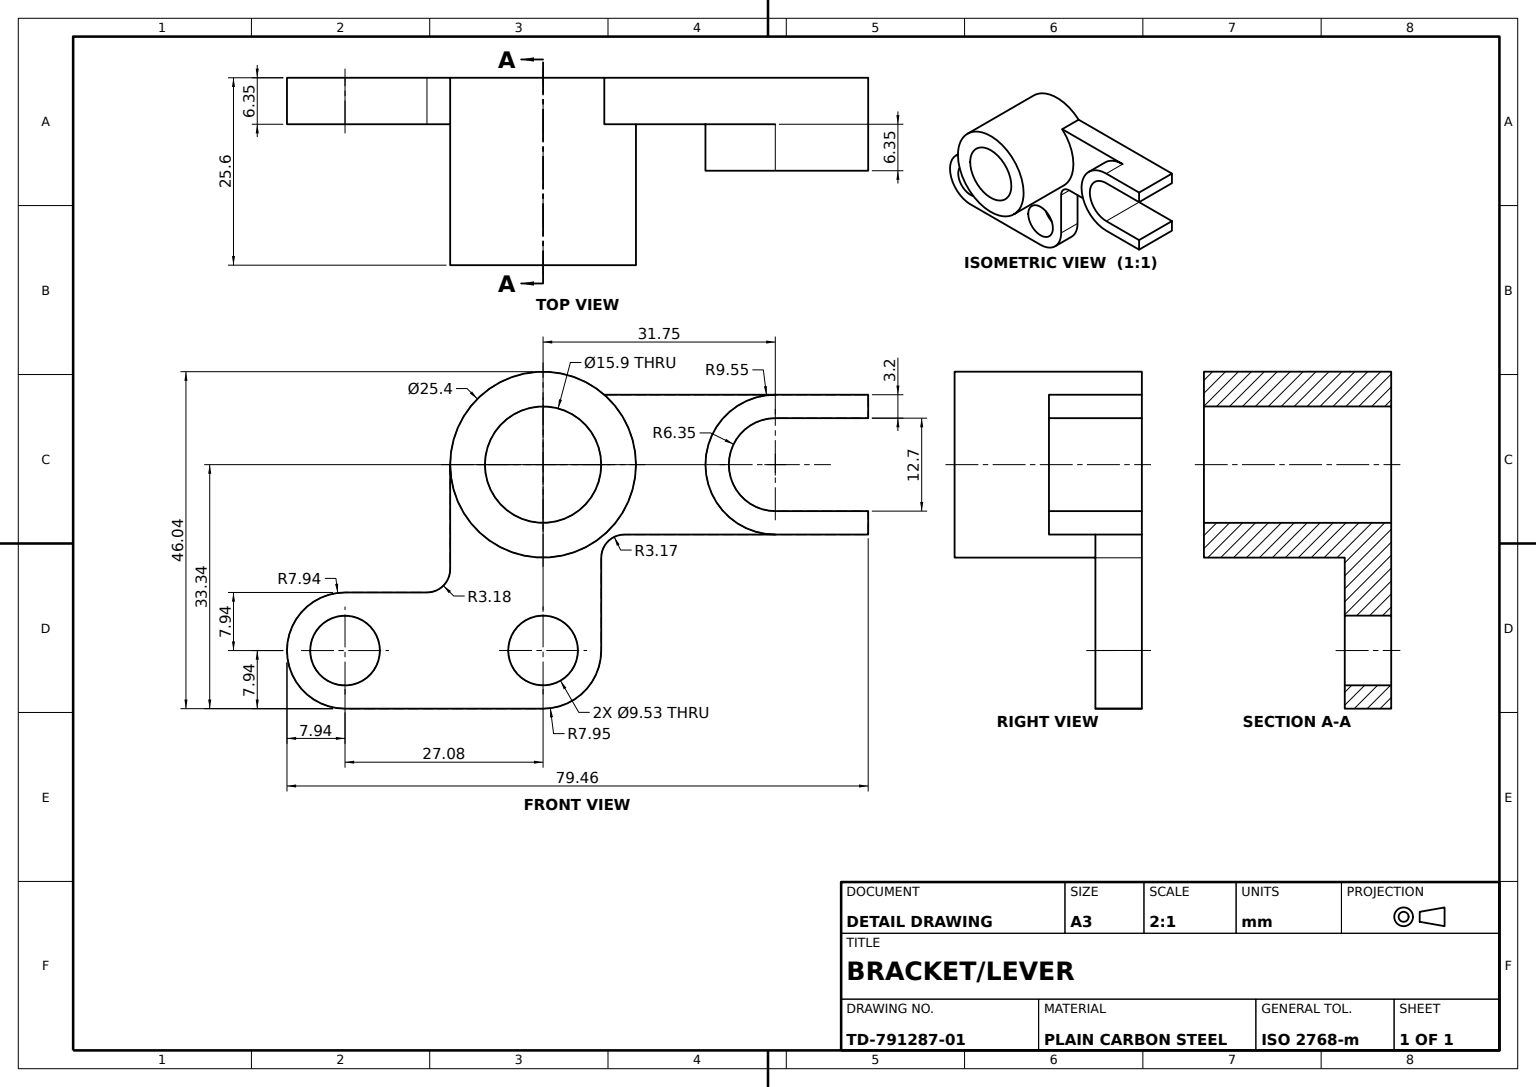
SolidWorks part; units mm, degrees
material "Plain Carbon Steel"
ref_plane "Front Plane" through (0, 0, 0) normal (0, 0, 1) x (1, 0, 0)
ref_plane "Top Plane" through (0, 0, 0) normal (0, 1, 0) x (1, 0, 0)
ref_plane "Right Plane" through (0, 0, 0) normal (1, 0, 0) x (0, 0, -1)
sketch "Hub Tube Sketch" plane through (0, 0, 0) normal (0, 0, 1) x (1, 0, 0)
  circle A0 centre (0, 0) radius 12.7
  circle A1 centre (0, 0) radius 7.9502
  dimension "D1" = 25.4
  dimension "D2" = 15.9004
extrude "Hub Tube" add sketch "Hub Tube Sketch" along normal blind 25.6032
sketch "Web Boss Sketch" plane through (0, 0, 0) normal (0, 0, 1) x (1, 0, 0)
  line L0 (31.75, 9.5504) -> (44.45, 9.5504)
  line L1 (44.45, 9.5504) -> (44.45, 6.35)
  line L2 (44.45, 6.35) -> (31.75, 6.35)
  line L3 (31.75, -6.35) -> (44.45, -6.35)
  line L4 (44.45, -6.35) -> (44.45, -9.5504)
  line L5 (44.45, -9.5504) -> (31.75, -9.5504)
  arc A0 (31.75, 9.5504) -> (31.75, -9.5504) centre (31.75, 0) ccw
  arc A1 (31.75, 6.35) -> (31.75, -6.35) centre (31.75, 0) ccw
  dimension "D1" = 12.7
  dimension "D2" = 12.7
  dimension "D3" = 3.2004
  dimension "D4" = 31.75
extrude "Web Boss" add sketch "Web Boss Sketch" along normal blind 12.7 separate body
sketch "Fork Ears Sketch" plane through (0, 0, 0) normal (0, 0, 1) x (1, 0, 0)
  line L0 (-12.7, 0) -> (-12.7, -14.2875)
  line L1 (-15.875, -17.4625) -> (-27.0764, -17.4625)
  line L2 (-27.0764, -33.3375) -> (0, -33.3375)
  line L3 (7.9502, -25.3873) -> (7.9502, -12.7254)
  line L4 (11.1252, -9.5504) -> (31.75, -9.5504)
  line L6 (31.75, 9.5504) -> (8.3714, 9.5504)
  circle A0 centre (0, 0) radius 12.7 construction
  arc A1 (-27.0764, -17.4625) -> (-27.0764, -33.3375) centre (-27.0764, -25.4) ccw
  arc A2 (31.75, 9.5504) -> (31.75, -9.5504) centre (31.75, 0) ccw construction
  circle A3 centre (-27.0764, -25.4) radius 4.7625
  arc A4 (0, -33.3375) -> (7.9502, -25.3873) centre (0, -25.3873) ccw
  arc A5 (7.9502, -12.7254) -> (11.1252, -9.5504) centre (11.1252, -12.7254) cw
  circle A6 centre (0, -25.3873) radius 4.7625
  arc A7 (-12.7, -14.2875) -> (-15.875, -17.4625) centre (-15.875, -14.2875) cw
  arc A8 (31.75, 9.5504) -> (31.75, -9.5504) centre (31.75, 0) ccw
  arc A10 (-12.7, 0) -> (8.3714, 9.5504) centre (0, 0) ccw
  dimension "D1" = 7.9375
  dimension "D2" = 9.525
  dimension "D3" = 7.9502
  dimension "D4" = 3.175
  dimension "D5" = 27.0764
  dimension "D8" = 3.175
  dimension "D6" = 25.4
  dimension "D7" = 31.75
extrude "Fork Ears" add sketch "Fork Ears Sketch" along normal blind 6.35
